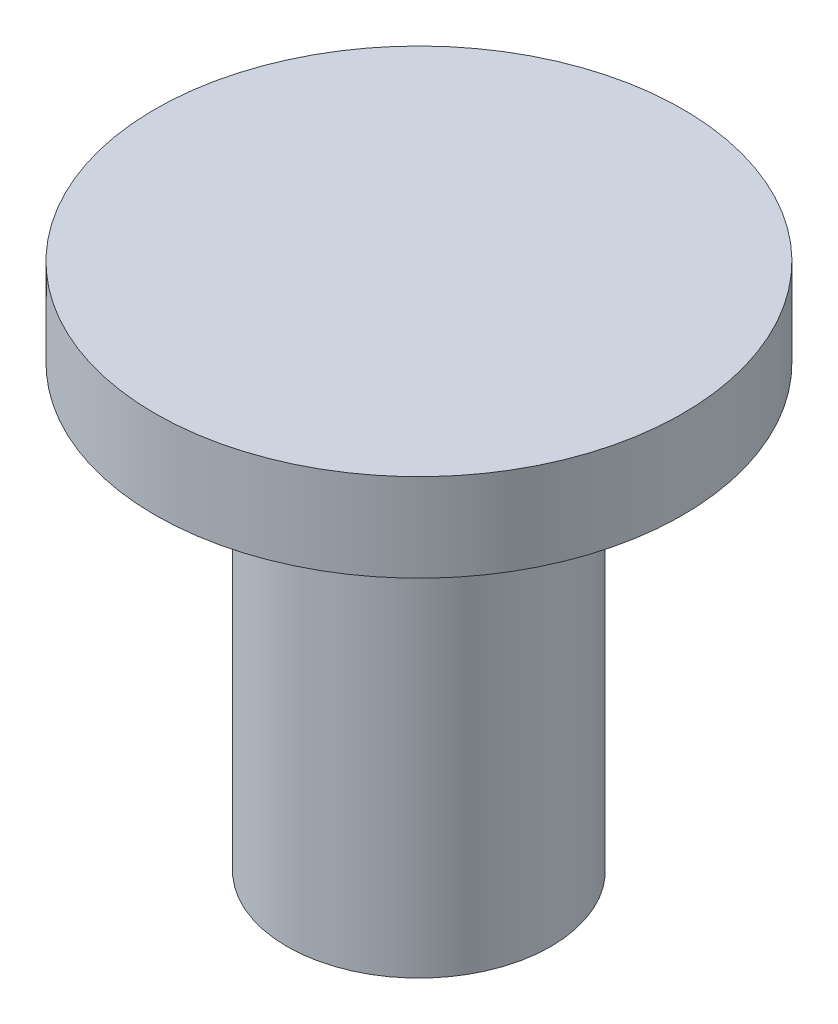
ISO-10303-21;
HEADER;
FILE_DESCRIPTION(('STEP AP214'),'2;1');
FILE_NAME('part.step','',(''),(''),'','','');
FILE_SCHEMA(('AUTOMOTIVE_DESIGN { 1 0 10303 214 1 1 1 1 }'));
ENDSEC;
DATA;
#1=APPLICATION_CONTEXT('core data for automotive mechanical design processes');
#2=APPLICATION_PROTOCOL_DEFINITION('international standard','automotive_design',2000,#1);
#3=PRODUCT_CONTEXT('',#1,'mechanical');
#4=PRODUCT('Part','Part','',(#3));
#5=PRODUCT_RELATED_PRODUCT_CATEGORY('part','',(#4));
#6=PRODUCT_DEFINITION_FORMATION('','',#4);
#7=PRODUCT_DEFINITION_CONTEXT('part definition',#1,'design');
#8=PRODUCT_DEFINITION('design','',#6,#7);
#9=PRODUCT_DEFINITION_SHAPE('','',#8);
#10=(LENGTH_UNIT() NAMED_UNIT(*) SI_UNIT(.MILLI.,.METRE.));
#11=(NAMED_UNIT(*) PLANE_ANGLE_UNIT() SI_UNIT($,.RADIAN.));
#12=(NAMED_UNIT(*) SI_UNIT($,.STERADIAN.) SOLID_ANGLE_UNIT());
#13=UNCERTAINTY_MEASURE_WITH_UNIT(LENGTH_MEASURE(1.E-05),#10,'distance_accuracy_value','');
#14=(GEOMETRIC_REPRESENTATION_CONTEXT(3) GLOBAL_UNCERTAINTY_ASSIGNED_CONTEXT((#13)) GLOBAL_UNIT_ASSIGNED_CONTEXT((#10,
#11,#12)) REPRESENTATION_CONTEXT('',''));
#15=CARTESIAN_POINT('',(0.,0.,0.));
#16=DIRECTION('',(0.,0.,1.));
#17=DIRECTION('',(1.,0.,0.));
#18=AXIS2_PLACEMENT_3D('',#15,#16,#17);
#19=CARTESIAN_POINT('',(0.,10.,0.));
#20=DIRECTION('',(0.,-1.,0.));
#21=DIRECTION('',(0.,0.,-1.));
#22=AXIS2_PLACEMENT_3D('',#19,#20,#21);
#23=CYLINDRICAL_SURFACE('',#22,3.);
#24=CARTESIAN_POINT('',(0.,10.,0.));
#25=DIRECTION('',(0.,1.,0.));
#26=DIRECTION('',(0.,0.,1.));
#27=AXIS2_PLACEMENT_3D('',#24,#25,#26);
#28=CIRCLE('',#27,3.);
#29=CARTESIAN_POINT('',(0.,10.,3.));
#30=VERTEX_POINT('',#29);
#31=EDGE_CURVE('E10',#30,#30,#28,.T.);
#32=ORIENTED_EDGE('',*,*,#31,.F.);
#33=EDGE_LOOP('',(#32));
#34=FACE_BOUND('',#33,.T.);
#35=CARTESIAN_POINT('',(0.,0.,0.));
#36=DIRECTION('',(0.,1.,0.));
#37=DIRECTION('',(0.,0.,1.));
#38=AXIS2_PLACEMENT_3D('',#35,#36,#37);
#39=CIRCLE('',#38,3.);
#40=CARTESIAN_POINT('',(0.,0.,3.));
#41=VERTEX_POINT('',#40);
#42=EDGE_CURVE('E45',#41,#41,#39,.T.);
#43=ORIENTED_EDGE('',*,*,#42,.T.);
#44=EDGE_LOOP('',(#43));
#45=FACE_BOUND('',#44,.T.);
#46=ADVANCED_FACE('F39',(#34,#45),#23,.T.);
#47=CARTESIAN_POINT('',(0.,0.,0.));
#48=DIRECTION('',(0.,1.,0.));
#49=DIRECTION('',(0.,0.,1.));
#50=AXIS2_PLACEMENT_3D('',#47,#48,#49);
#51=PLANE('',#50);
#52=ORIENTED_EDGE('',*,*,#42,.F.);
#53=EDGE_LOOP('',(#52));
#54=FACE_BOUND('',#53,.T.);
#55=ADVANCED_FACE('F65',(#54),#51,.F.);
#56=CARTESIAN_POINT('',(0.,12.,0.));
#57=DIRECTION('',(0.,-1.,0.));
#58=DIRECTION('',(0.,0.,-1.));
#59=AXIS2_PLACEMENT_3D('',#56,#57,#58);
#60=CYLINDRICAL_SURFACE('',#59,6.);
#61=CARTESIAN_POINT('',(0.,12.,0.));
#62=DIRECTION('',(0.,1.,0.));
#63=DIRECTION('',(0.,0.,1.));
#64=AXIS2_PLACEMENT_3D('',#61,#62,#63);
#65=CIRCLE('',#64,6.);
#66=CARTESIAN_POINT('',(0.,12.,6.));
#67=VERTEX_POINT('',#66);
#68=EDGE_CURVE('E47',#67,#67,#65,.T.);
#69=ORIENTED_EDGE('',*,*,#68,.F.);
#70=EDGE_LOOP('',(#69));
#71=FACE_BOUND('',#70,.T.);
#72=CARTESIAN_POINT('',(0.,10.,0.));
#73=DIRECTION('',(0.,1.,0.));
#74=DIRECTION('',(0.,0.,1.));
#75=AXIS2_PLACEMENT_3D('',#72,#73,#74);
#76=CIRCLE('',#75,6.);
#77=CARTESIAN_POINT('',(0.,10.,6.));
#78=VERTEX_POINT('',#77);
#79=EDGE_CURVE('E51',#78,#78,#76,.T.);
#80=ORIENTED_EDGE('',*,*,#79,.T.);
#81=EDGE_LOOP('',(#80));
#82=FACE_BOUND('',#81,.T.);
#83=ADVANCED_FACE('F56',(#71,#82),#60,.T.);
#84=CARTESIAN_POINT('',(0.,12.,0.));
#85=DIRECTION('',(0.,1.,0.));
#86=DIRECTION('',(0.,0.,1.));
#87=AXIS2_PLACEMENT_3D('',#84,#85,#86);
#88=PLANE('',#87);
#89=ORIENTED_EDGE('',*,*,#68,.T.);
#90=EDGE_LOOP('',(#89));
#91=FACE_BOUND('',#90,.T.);
#92=ADVANCED_FACE('F60',(#91),#88,.T.);
#93=CARTESIAN_POINT('',(0.,10.,0.));
#94=DIRECTION('',(0.,1.,0.));
#95=DIRECTION('',(0.,0.,1.));
#96=AXIS2_PLACEMENT_3D('',#93,#94,#95);
#97=PLANE('',#96);
#98=ORIENTED_EDGE('',*,*,#31,.T.);
#99=EDGE_LOOP('',(#98));
#100=FACE_BOUND('',#99,.T.);
#101=ORIENTED_EDGE('',*,*,#79,.F.);
#102=EDGE_LOOP('',(#101));
#103=FACE_BOUND('',#102,.T.);
#104=ADVANCED_FACE('F66',(#100,#103),#97,.F.);
#105=CLOSED_SHELL('',(#46,#55,#83,#92,#104));
#106=MANIFOLD_SOLID_BREP('B2',#105);
#107=ADVANCED_BREP_SHAPE_REPRESENTATION('',(#18,#106),#14);
#108=SHAPE_DEFINITION_REPRESENTATION(#9,#107);
ENDSEC;
END-ISO-10303-21;
